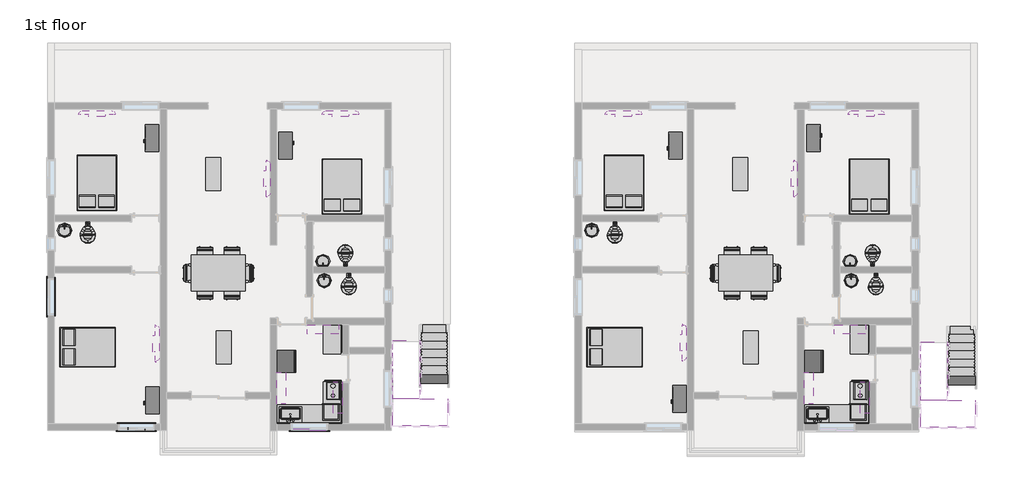
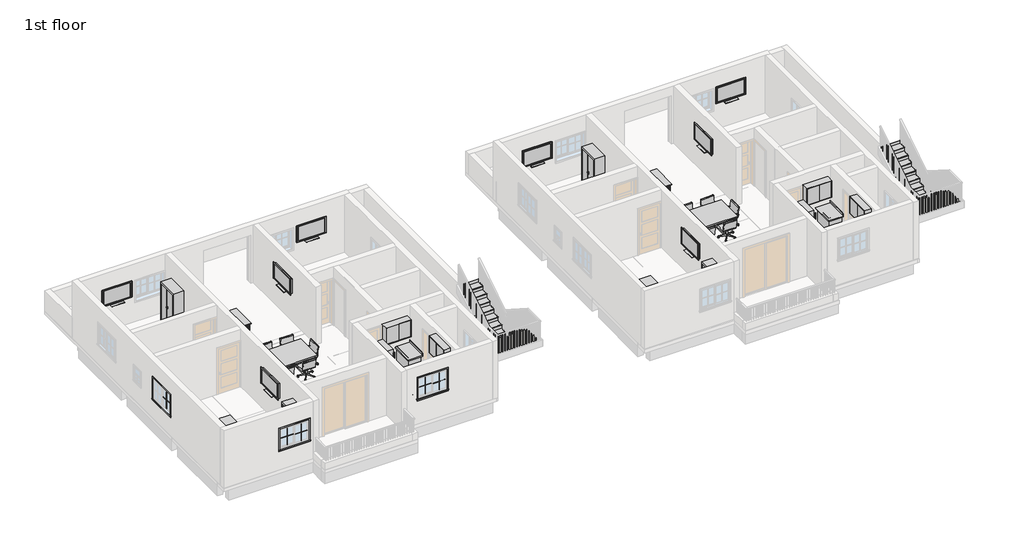
# One storey, part 7 of 8: 56 furniture elements, 24 proxies, 14 flow terminals, 4 stair flights, 2 slabs.
"""IFC4 building model written with IfcOpenShell, lengths in millimetres."""

from ifc_helpers import new_model, si_unit, origin, place, context, project, spatial, transform, mapped, element, save
from components import proxy_3c1fa1d0, proxy_caef4acf, muntin_pattern_2x2_muntin_pattern_2x2_0ac132d2, muntin_pattern_2x2_muntin_pattern_2x2_1fb5fae3, proxy_68898770, proxy_19935bb1, trim_window_exterior_flat_with_sill_c4e67c73, trim_window_exterior_flat_with_sill_729ce974, trim_window_interior_flat_picture_frame_cf1733af, trim_window_interior_flat_picture_frame_5593adf3, flow_terminal_4d548711, flow_terminal_a43f4bde, flow_terminal_3100e559, furniture_6369f5ad, furniture_f415afdb, furniture_97fe820d, furniture_b58f7881, furniture_d3d70ab1, chair_task_chair_task_b7f3823b, chair_task_arms_chair_task_arms_fa5a08ef, furniture_47cc8d9a, furniture_d87d408b, furniture_e7d75d8c, furniture_0b81fedb, furniture_74675f9f, furniture_0bcc43ae, upper_cabinet_sliding_double_door_wall_3e092c2a, non_monolithic_landing_27542c2d, non_monolithic_landing_419a9ad9, stair_flight_dc742093, stair_flight_4d250dde, stair_flight_731070e0, stair_flight_a0137449

model = new_model("IFC4")

# Units and contexts
model_context = context("Model", 3, world=origin())
ifc_project = project(units=[si_unit("LENGTHUNIT", "METRE", prefix="MILLI")], contexts=[model_context])

# Site, building, storey
site = spatial("IfcSite", under=ifc_project)
building = spatial("IfcBuilding", under=site)
storey = spatial("IfcBuildingStorey", under=building, Name="1st floor", Elevation=3810.0)

# Proxies
placement = place(None, origin())
proxy_shape = proxy_3c1fa1d0(model_context)
element("IfcBuildingElementProxy", 1, Name="Cook Top-2 Unit : 12\" x 18\" 2", ObjectType="Cook Top-2 Unit : 12\" x 18\" 2", at=placement, inside=storey, context=model_context, shape_type="MappedRepresentation", body=[
    mapped(proxy_shape, transform((-6699.3993763, -3292.5061971, 3810.0), x_axis=(1.0, 0.0, 0.0), y_axis=(0.0, 1.0, 0.0), z_axis=(0.0, 0.0, 1.0))),
])
element("IfcBuildingElementProxy", 2, Name="Cook Top-2 Unit : 12\" x 18\" 2", ObjectType="Cook Top-2 Unit : 12\" x 18\" 2", at=placement, inside=storey, context=model_context, shape_type="MappedRepresentation", body=[
    mapped(proxy_shape, transform((11175.1761273, -3292.5061971, 3810.0), x_axis=(1.0, 0.0, 0.0), y_axis=(0.0, 1.0, 0.0), z_axis=(0.0, 0.0, 1.0))),
])
proxy_2_shape = proxy_caef4acf(model_context)
element("IfcBuildingElementProxy", 3, Name="Cook Top-2 Unit : 16\" x 22\"", ObjectType="Cook Top-2 Unit : 16\" x 22\"", at=placement, inside=storey, context=model_context, shape_type="MappedRepresentation", body=[
    mapped(proxy_2_shape, transform((-6775.5993763, -4038.6311971, 3810.0), x_axis=(1.0, 0.0, 0.0), y_axis=(0.0, 1.0, 0.0), z_axis=(0.0, 0.0, 1.0))),
])
element("IfcBuildingElementProxy", 4, Name="Cook Top-2 Unit : 16\" x 22\"", ObjectType="Cook Top-2 Unit : 16\" x 22\"", at=placement, inside=storey, context=model_context, shape_type="MappedRepresentation", body=[
    mapped(proxy_2_shape, transform((-6864.4993763, -4089.4311971, 3810.0), x_axis=(1.0, 0.0, 0.0), y_axis=(0.0, 1.0, 0.0), z_axis=(0.0, 0.0, 1.0))),
])
element("IfcBuildingElementProxy", 5, Name="Cook Top-2 Unit : 16\" x 22\"", ObjectType="Cook Top-2 Unit : 16\" x 22\"", at=placement, inside=storey, context=model_context, shape_type="MappedRepresentation", body=[
    mapped(proxy_2_shape, transform((-6699.3993763, -3340.1311971, 3810.0), x_axis=(1.0, 0.0, 0.0), y_axis=(0.0, 1.0, 0.0), z_axis=(0.0, 0.0, 1.0))),
])
element("IfcBuildingElementProxy", 6, Name="Cook Top-2 Unit : 16\" x 22\"", ObjectType="Cook Top-2 Unit : 16\" x 22\"", at=placement, inside=storey, context=model_context, shape_type="MappedRepresentation", body=[
    mapped(proxy_2_shape, transform((-6737.4993763, -3556.0311971, 3810.0), x_axis=(1.0, 0.0, 0.0), y_axis=(0.0, 1.0, 0.0), z_axis=(0.0, 0.0, 1.0))),
])
element("IfcBuildingElementProxy", 7, Name="Cook Top-2 Unit : 16\" x 22\"", ObjectType="Cook Top-2 Unit : 16\" x 22\"", at=placement, inside=storey, context=model_context, shape_type="MappedRepresentation", body=[
    mapped(proxy_2_shape, transform((11098.9761273, -4038.6311971, 3810.0), x_axis=(1.0, 0.0, 0.0), y_axis=(0.0, 1.0, 0.0), z_axis=(0.0, 0.0, 1.0))),
])
element("IfcBuildingElementProxy", 8, Name="Cook Top-2 Unit : 16\" x 22\"", ObjectType="Cook Top-2 Unit : 16\" x 22\"", at=placement, inside=storey, context=model_context, shape_type="MappedRepresentation", body=[
    mapped(proxy_2_shape, transform((11010.0761273, -4089.4311971, 3810.0), x_axis=(1.0, 0.0, 0.0), y_axis=(0.0, 1.0, 0.0), z_axis=(0.0, 0.0, 1.0))),
])
element("IfcBuildingElementProxy", 9, Name="Cook Top-2 Unit : 16\" x 22\"", ObjectType="Cook Top-2 Unit : 16\" x 22\"", at=placement, inside=storey, context=model_context, shape_type="MappedRepresentation", body=[
    mapped(proxy_2_shape, transform((11175.1761273, -3340.1311971, 3810.0), x_axis=(1.0, 0.0, 0.0), y_axis=(0.0, 1.0, 0.0), z_axis=(0.0, 0.0, 1.0))),
])
element("IfcBuildingElementProxy", 10, Name="Cook Top-2 Unit : 16\" x 22\"", ObjectType="Cook Top-2 Unit : 16\" x 22\"", at=placement, inside=storey, context=model_context, shape_type="MappedRepresentation", body=[
    mapped(proxy_2_shape, transform((11137.0761273, -3556.0311971, 3810.0), x_axis=(1.0, 0.0, 0.0), y_axis=(0.0, 1.0, 0.0), z_axis=(0.0, 0.0, 1.0))),
])
muntin_pattern_2x2_muntin_pattern_2x2_shape = muntin_pattern_2x2_muntin_pattern_2x2_0ac132d2(model_context)
element("IfcBuildingElementProxy", 11, Name="Muntin Pattern_2x2 : Muntin Pattern_2x2", ObjectType="Muntin Pattern_2x2 : Muntin Pattern_2x2", at=placement, inside=storey, context=model_context, shape_type="MappedRepresentation", body=[
    mapped(muntin_pattern_2x2_muntin_pattern_2x2_shape, transform((-7707.4618763, -4551.3314015, 5035.55), x_axis=(-1.0, 0.0, 0.0), y_axis=(0.0, -1.0, 0.0), z_axis=(0.0, 0.0, 1.0))),
])
element("IfcBuildingElementProxy", 12, Name="Muntin Pattern_2x2 : Muntin Pattern_2x2", ObjectType="Muntin Pattern_2x2 : Muntin Pattern_2x2", at=placement, inside=storey, context=model_context, shape_type="MappedRepresentation", body=[
    mapped(muntin_pattern_2x2_muntin_pattern_2x2_shape, transform((-7139.1368763, -4595.7814015, 5035.55), x_axis=(-1.0, 0.0, 0.0), y_axis=(0.0, -1.0, 0.0), z_axis=(0.0, 0.0, 1.0))),
])
element("IfcBuildingElementProxy", 13, Name="Muntin Pattern_2x2 : Muntin Pattern_2x2", ObjectType="Muntin Pattern_2x2 : Muntin Pattern_2x2", at=placement, inside=storey, context=model_context, shape_type="MappedRepresentation", body=[
    mapped(muntin_pattern_2x2_muntin_pattern_2x2_shape, transform((-13574.8618763, -4551.3314015, 4806.95), x_axis=(-1.0, 0.0, 0.0), y_axis=(0.0, -1.0, 0.0), z_axis=(0.0, 0.0, 1.0))),
])
element("IfcBuildingElementProxy", 14, Name="Muntin Pattern_2x2 : Muntin Pattern_2x2", ObjectType="Muntin Pattern_2x2 : Muntin Pattern_2x2", at=placement, inside=storey, context=model_context, shape_type="MappedRepresentation", body=[
    mapped(muntin_pattern_2x2_muntin_pattern_2x2_shape, transform((-13006.5368763, -4595.7814015, 4806.95), x_axis=(-1.0, 0.0, 0.0), y_axis=(0.0, -1.0, 0.0), z_axis=(0.0, 0.0, 1.0))),
])
muntin_pattern_2x2_muntin_pattern_2x2_2_shape = muntin_pattern_2x2_muntin_pattern_2x2_1fb5fae3(model_context)
element("IfcBuildingElementProxy", 15, Name="Muntin Pattern_2x2 : Muntin Pattern_2x2", ObjectType="Muntin Pattern_2x2 : Muntin Pattern_2x2", at=placement, inside=storey, context=model_context, shape_type="MappedRepresentation", body=[
    mapped(muntin_pattern_2x2_muntin_pattern_2x2_2_shape, transform((-16246.6243763, -355.5689015, 4806.95), x_axis=(0.0, -1.0, 0.0), y_axis=(1.0, 0.0, 0.0), z_axis=(0.0, 0.0, 1.0))),
])
proxy_3_shape = proxy_68898770(model_context)
element("IfcBuildingElementProxy", 16, Name="Oven Single-Built-in : 21\" x 23 1/2\" x 21\"", ObjectType="Oven Single-Built-in : 21\" x 23 1/2\" x 21\"", at=placement, inside=storey, context=model_context, shape_type="MappedRepresentation", body=[
    mapped(proxy_3_shape, transform((-6728.2243036, -3854.6405426, 4622.8), x_axis=(-1.0, 0.0, 0.0), y_axis=(0.0, -1.0, 0.0), z_axis=(0.0, 0.0, 1.0))),
])
element("IfcBuildingElementProxy", 17, Name="Oven Single-Built-in : 21\" x 23 1/2\" x 21\"", ObjectType="Oven Single-Built-in : 21\" x 23 1/2\" x 21\"", at=placement, inside=storey, context=model_context, shape_type="MappedRepresentation", body=[
    mapped(proxy_3_shape, transform((11146.3512, -3854.6405426, 4622.8), x_axis=(-1.0, 0.0, 0.0), y_axis=(0.0, -1.0, 0.0), z_axis=(0.0, 0.0, 1.0))),
])
proxy_4_shape = proxy_19935bb1(model_context)
element("IfcBuildingElementProxy", 18, Name="Refrigerator-Built-in : 30\" x 24\" LH", ObjectType="Refrigerator-Built-in : 30\" x 24\" LH", at=placement, inside=storey, context=model_context, shape_type="MappedRepresentation", body=[
    mapped(proxy_4_shape, transform((-8238.0754048, -2262.1564015, 3810.0), x_axis=(0.0, 1.0, 0.0), y_axis=(-1.0, 0.0, 0.0), z_axis=(0.0, 0.0, 1.0))),
])
element("IfcBuildingElementProxy", 19, Name="Refrigerator-Built-in : 30\" x 24\" LH", ObjectType="Refrigerator-Built-in : 30\" x 24\" LH", at=placement, inside=storey, context=model_context, shape_type="MappedRepresentation", body=[
    mapped(proxy_4_shape, transform((9636.5000988, -2262.1564015, 3810.0), x_axis=(0.0, 1.0, 0.0), y_axis=(-1.0, 0.0, 0.0), z_axis=(0.0, 0.0, 1.0))),
])
trim_window_exterior_flat_with_sill_shape = trim_window_exterior_flat_with_sill_c4e67c73(model_context)
element("IfcBuildingElementProxy", 20, Name="Trim-Window-Exterior-Flat : with Sill", ObjectType="Trim-Window-Exterior-Flat : with Sill", at=placement, inside=storey, context=model_context, shape_type="MappedRepresentation", body=[
    mapped(trim_window_exterior_flat_with_sill_shape, transform((-7423.2993763, -4605.3064015, 5867.4), x_axis=(1.0, 0.0, 0.0), y_axis=(0.0, 0.0, 1.0), z_axis=(0.0, -1.0, 0.0))),
])
element("IfcBuildingElementProxy", 21, Name="Trim-Window-Exterior-Flat : with Sill", ObjectType="Trim-Window-Exterior-Flat : with Sill", at=placement, inside=storey, context=model_context, shape_type="MappedRepresentation", body=[
    mapped(trim_window_exterior_flat_with_sill_shape, transform((-13290.6993763, -4605.3064015, 5638.8), x_axis=(1.0, 0.0, 0.0), y_axis=(0.0, 0.0, 1.0), z_axis=(0.0, -1.0, 0.0))),
])
trim_window_exterior_flat_with_sill_2_shape = trim_window_exterior_flat_with_sill_729ce974(model_context)
element("IfcBuildingElementProxy", 22, Name="Trim-Window-Exterior-Flat : with Sill", ObjectType="Trim-Window-Exterior-Flat : with Sill", at=placement, inside=storey, context=model_context, shape_type="MappedRepresentation", body=[
    mapped(trim_window_exterior_flat_with_sill_2_shape, transform((-16300.5993763, -71.4064015, 5638.8), x_axis=(0.0, 1.0, 0.0), y_axis=(0.0, 0.0, -1.0), z_axis=(-1.0, 0.0, 0.0))),
])
trim_window_interior_flat_picture_frame_shape = trim_window_interior_flat_picture_frame_cf1733af(model_context)
element("IfcBuildingElementProxy", 23, Name="Trim-Window-Interior-Flat : Picture Frame", ObjectType="Trim-Window-Interior-Flat : Picture Frame", at=placement, inside=storey, context=model_context, shape_type="MappedRepresentation", body=[
    mapped(trim_window_interior_flat_picture_frame_shape, transform((-13290.6993763, -4376.7064015, 5638.8), x_axis=(-1.0, 0.0, 0.0), y_axis=(0.0, 0.0, 1.0), z_axis=(0.0, 1.0, 0.0))),
])
trim_window_interior_flat_picture_frame_2_shape = trim_window_interior_flat_picture_frame_5593adf3(model_context)
element("IfcBuildingElementProxy", 24, Name="Trim-Window-Interior-Flat : Picture Frame", ObjectType="Trim-Window-Interior-Flat : Picture Frame", at=placement, inside=storey, context=model_context, shape_type="MappedRepresentation", body=[
    mapped(trim_window_interior_flat_picture_frame_2_shape, transform((-16071.9993763, -71.4064015, 5638.8), x_axis=(0.0, -1.0, 0.0), y_axis=(0.0, 0.0, -1.0), z_axis=(1.0, 0.0, 0.0))),
])

# Flow terminals
flow_terminal_shape = flow_terminal_4d548711(model_context)
element("IfcFlowTerminal", 25, ObjectType="Sink Kitchen-Single : 30\" x 21\"", at=placement, inside=storey, context=model_context, shape_type="MappedRepresentation", body=[
    mapped(flow_terminal_shape, transform((-8055.3101357, -4069.5610004, 3810.0), x_axis=(-1.0, 0.0, 0.0), y_axis=(0.0, -1.0, 0.0), z_axis=(0.0, 0.0, 1.0))),
])
element("IfcFlowTerminal", 26, ObjectType="Sink Kitchen-Single : 30\" x 21\"", at=placement, inside=storey, context=model_context, shape_type="MappedRepresentation", body=[
    mapped(flow_terminal_shape, transform((9819.2653679, -4069.5610004, 3810.0), x_axis=(-1.0, 0.0, 0.0), y_axis=(0.0, -1.0, 0.0), z_axis=(0.0, 0.0, 1.0))),
])
flow_terminal_2_shape = flow_terminal_a43f4bde(model_context)
element("IfcFlowTerminal", 27, ObjectType="Sink Vanity-Round : 19\" x 19\"", at=placement, inside=storey, context=model_context, shape_type="MappedRepresentation", body=[
    mapped(flow_terminal_2_shape, transform((-15825.7511169, 2099.027665, 3810.0), x_axis=(1.0, 0.0, 0.0), y_axis=(0.0, 1.0, 0.0), z_axis=(0.0, 0.0, 1.0))),
])
element("IfcFlowTerminal", 28, ObjectType="Sink Vanity-Round : 19\" x 19\"", at=placement, inside=storey, context=model_context, shape_type="MappedRepresentation", body=[
    mapped(flow_terminal_2_shape, transform((-6868.8660625, 1205.7175518, 3810.0), x_axis=(-0.999964486635994, 0.008427660815032186, 0.0), y_axis=(-0.008427660815032186, -0.999964486635994, 0.0), z_axis=(0.0, 0.0, 1.0))),
])
element("IfcFlowTerminal", 29, ObjectType="Sink Vanity-Round : 19\" x 19\"", at=placement, inside=storey, context=model_context, shape_type="MappedRepresentation", body=[
    mapped(flow_terminal_2_shape, transform((-7024.6511169, 390.0887767, 3810.0), x_axis=(1.0, 0.0, 0.0), y_axis=(0.0, 1.0, 0.0), z_axis=(0.0, 0.0, 1.0))),
])
element("IfcFlowTerminal", 30, ObjectType="Sink Vanity-Round : 19\" x 19\"", at=placement, inside=storey, context=model_context, shape_type="MappedRepresentation", body=[
    mapped(flow_terminal_2_shape, transform((2048.8243868, 2099.027665, 3810.0), x_axis=(1.0, 0.0, 0.0), y_axis=(0.0, 1.0, 0.0), z_axis=(0.0, 0.0, 1.0))),
])
element("IfcFlowTerminal", 31, ObjectType="Sink Vanity-Round : 19\" x 19\"", at=placement, inside=storey, context=model_context, shape_type="MappedRepresentation", body=[
    mapped(flow_terminal_2_shape, transform((11005.7094411, 1205.7175518, 3810.0), x_axis=(-0.999964486635994, 0.008427660815032186, 0.0), y_axis=(-0.008427660815032186, -0.999964486635994, 0.0), z_axis=(0.0, 0.0, 1.0))),
])
element("IfcFlowTerminal", 32, ObjectType="Sink Vanity-Round : 19\" x 19\"", at=placement, inside=storey, context=model_context, shape_type="MappedRepresentation", body=[
    mapped(flow_terminal_2_shape, transform((10849.9243868, 390.0887767, 3810.0), x_axis=(1.0, 0.0, 0.0), y_axis=(0.0, 1.0, 0.0), z_axis=(0.0, 0.0, 1.0))),
])
flow_terminal_3_shape = flow_terminal_3100e559(model_context)
element("IfcFlowTerminal", 33, ObjectType="Toilet-Commercial-Wall-3D : 15\" Seat Height", at=placement, inside=storey, context=model_context, shape_type="MappedRepresentation", body=[
    mapped(flow_terminal_3_shape, transform((-5684.8962225, 842.9935985, 3810.0), x_axis=(-1.0, 0.0, 0.0), y_axis=(0.0, -1.0, 0.0), z_axis=(0.0, 0.0, 1.0))),
])
element("IfcFlowTerminal", 34, ObjectType="Toilet-Commercial-Wall-3D : 15\" Seat Height", at=placement, inside=storey, context=model_context, shape_type="MappedRepresentation", body=[
    mapped(flow_terminal_3_shape, transform((-6609.0025301, 842.9935985, 3810.0), x_axis=(1.0, 0.0, 0.0), y_axis=(0.0, 1.0, 0.0), z_axis=(0.0, 0.0, 1.0))),
])
element("IfcFlowTerminal", 35, ObjectType="Toilet-Commercial-Wall-3D : 15\" Seat Height", at=placement, inside=storey, context=model_context, shape_type="MappedRepresentation", body=[
    mapped(flow_terminal_3_shape, transform((-14536.7962225, 2595.5935985, 3810.0), x_axis=(-1.0, 0.0, 0.0), y_axis=(0.0, -1.0, 0.0), z_axis=(0.0, 0.0, 1.0))),
])
element("IfcFlowTerminal", 36, ObjectType="Toilet-Commercial-Wall-3D : 15\" Seat Height", at=placement, inside=storey, context=model_context, shape_type="MappedRepresentation", body=[
    mapped(flow_terminal_3_shape, transform((12189.6792812, 842.9935985, 3810.0), x_axis=(-1.0, 0.0, 0.0), y_axis=(0.0, -1.0, 0.0), z_axis=(0.0, 0.0, 1.0))),
])
element("IfcFlowTerminal", 37, ObjectType="Toilet-Commercial-Wall-3D : 15\" Seat Height", at=placement, inside=storey, context=model_context, shape_type="MappedRepresentation", body=[
    mapped(flow_terminal_3_shape, transform((11265.5729735, 842.9935985, 3810.0), x_axis=(1.0, 0.0, 0.0), y_axis=(0.0, 1.0, 0.0), z_axis=(0.0, 0.0, 1.0))),
])
element("IfcFlowTerminal", 38, ObjectType="Toilet-Commercial-Wall-3D : 15\" Seat Height", at=placement, inside=storey, context=model_context, shape_type="MappedRepresentation", body=[
    mapped(flow_terminal_3_shape, transform((3337.7792812, 2595.5935985, 3810.0), x_axis=(-1.0, 0.0, 0.0), y_axis=(0.0, -1.0, 0.0), z_axis=(0.0, 0.0, 1.0))),
])

# Furniture
furniture_shape = furniture_6369f5ad(model_context)
element("IfcFurniture", 39, ObjectType="Base Cabinet-Acid Storage Unit : 30\" 2", at=placement, inside=storey, context=model_context, shape_type="MappedRepresentation", body=[
    mapped(furniture_shape, transform((-6343.7993763, -3202.2686966, 3810.0), x_axis=(0.0, -1.0, 0.0), y_axis=(1.0, 0.0, 0.0), z_axis=(0.0, 0.0, 1.0))),
])
element("IfcFurniture", 40, ObjectType="Base Cabinet-Acid Storage Unit : 30\" 2", at=placement, inside=storey, context=model_context, shape_type="MappedRepresentation", body=[
    mapped(furniture_shape, transform((11530.7761273, -3202.2686966, 3810.0), x_axis=(0.0, -1.0, 0.0), y_axis=(1.0, 0.0, 0.0), z_axis=(0.0, 0.0, 1.0))),
])
furniture_2_shape = furniture_f415afdb(model_context)
element("IfcFurniture", 41, ObjectType="Base Cabinet-Combo01 : 30\" 2", at=placement, inside=storey, context=model_context, shape_type="MappedRepresentation", body=[
    mapped(furniture_2_shape, transform((-6318.3993763, -1386.1686966, 3810.0), x_axis=(0.0, -1.0, 0.0), y_axis=(1.0, 0.0, 0.0), z_axis=(0.0, 0.0, 1.0))),
])
element("IfcFurniture", 42, ObjectType="Base Cabinet-Combo01 : 30\" 2", at=placement, inside=storey, context=model_context, shape_type="MappedRepresentation", body=[
    mapped(furniture_2_shape, transform((11556.1761273, -1386.1686966, 3810.0), x_axis=(0.0, -1.0, 0.0), y_axis=(1.0, 0.0, 0.0), z_axis=(0.0, 0.0, 1.0))),
])
furniture_3_shape = furniture_97fe820d(model_context)
element("IfcFurniture", 43, ObjectType="Base Cabinet-Corner Unit-Square : 36\"", at=placement, inside=storey, context=model_context, shape_type="MappedRepresentation", body=[
    mapped(furniture_3_shape, transform((-6318.3993763, -3849.9686966, 3810.0), x_axis=(0.0, -1.0, 0.0), y_axis=(1.0, 0.0, 0.0), z_axis=(0.0, 0.0, 1.0))),
])
element("IfcFurniture", 44, ObjectType="Base Cabinet-Corner Unit-Square : 36\"", at=placement, inside=storey, context=model_context, shape_type="MappedRepresentation", body=[
    mapped(furniture_3_shape, transform((11556.1761273, -3849.9686966, 3810.0), x_axis=(0.0, -1.0, 0.0), y_axis=(1.0, 0.0, 0.0), z_axis=(0.0, 0.0, 1.0))),
])
furniture_4_shape = furniture_b58f7881(model_context)
element("IfcFurniture", 45, ObjectType="Bed-Box : Double 53\" x 74\"", at=placement, inside=storey, context=model_context, shape_type="MappedRepresentation", body=[
    mapped(furniture_4_shape, transform((-14292.2379089, 3557.6185064, 3810.0), x_axis=(-1.0, 0.0, 0.0), y_axis=(0.0, -1.0, 0.0), z_axis=(0.0, 0.0, 1.0))),
])
element("IfcFurniture", 46, ObjectType="Bed-Box : Double 53\" x 74\"", at=placement, inside=storey, context=model_context, shape_type="MappedRepresentation", body=[
    mapped(furniture_4_shape, transform((-15182.9191795, -2125.0588605, 3810.0), x_axis=(0.0, 1.0, 0.0), y_axis=(-1.0, 0.0, 0.0), z_axis=(0.0, 0.0, 1.0))),
])
element("IfcFurniture", 47, ObjectType="Bed-Box : Double 53\" x 74\"", at=placement, inside=storey, context=model_context, shape_type="MappedRepresentation", body=[
    mapped(furniture_4_shape, transform((-5979.2469173, 3433.3274594, 3810.0), x_axis=(-1.0, 0.0, 0.0), y_axis=(0.0, -1.0, 0.0), z_axis=(0.0, 0.0, 1.0))),
])
element("IfcFurniture", 48, ObjectType="Bed-Box : Double 53\" x 74\"", at=placement, inside=storey, context=model_context, shape_type="MappedRepresentation", body=[
    mapped(furniture_4_shape, transform((3582.3375948, 3557.6185064, 3810.0), x_axis=(-1.0, 0.0, 0.0), y_axis=(0.0, -1.0, 0.0), z_axis=(0.0, 0.0, 1.0))),
])
element("IfcFurniture", 49, ObjectType="Bed-Box : Double 53\" x 74\"", at=placement, inside=storey, context=model_context, shape_type="MappedRepresentation", body=[
    mapped(furniture_4_shape, transform((2691.6563242, -2125.0588605, 3810.0), x_axis=(0.0, 1.0, 0.0), y_axis=(-1.0, 0.0, 0.0), z_axis=(0.0, 0.0, 1.0))),
])
element("IfcFurniture", 50, ObjectType="Bed-Box : Double 53\" x 74\"", at=placement, inside=storey, context=model_context, shape_type="MappedRepresentation", body=[
    mapped(furniture_4_shape, transform((11895.3285864, 3433.3274594, 3810.0), x_axis=(-1.0, 0.0, 0.0), y_axis=(0.0, -1.0, 0.0), z_axis=(0.0, 0.0, 1.0))),
])
furniture_5_shape = furniture_d3d70ab1(model_context)
element("IfcFurniture", 51, ObjectType="Cabinet-Storage : 36\" x 18\" x 72\"", at=placement, inside=storey, context=model_context, shape_type="MappedRepresentation", body=[
    mapped(furniture_5_shape, transform((-12757.2993763, 5305.7833167, 3810.0), x_axis=(0.0, -1.0, 0.0), y_axis=(1.0, 0.0, 0.0), z_axis=(0.0, 0.0, 1.0))),
])
element("IfcFurniture", 52, ObjectType="Cabinet-Storage : 36\" x 18\" x 72\"", at=placement, inside=storey, context=model_context, shape_type="MappedRepresentation", body=[
    mapped(furniture_5_shape, transform((-8236.2515468, 5059.3935985, 3810.0), x_axis=(0.0, 1.0, 0.0), y_axis=(-1.0, 0.0, 0.0), z_axis=(0.0, 0.0, 1.0))),
])
element("IfcFurniture", 53, ObjectType="Cabinet-Storage : 36\" x 18\" x 72\"", at=placement, inside=storey, context=model_context, shape_type="MappedRepresentation", body=[
    mapped(furniture_5_shape, transform((-12748.5420807, -3590.3671413, 3810.0), x_axis=(0.0, -1.0, 0.0), y_axis=(1.0, 0.0, 0.0), z_axis=(0.0, 0.0, 1.0))),
])
element("IfcFurniture", 54, ObjectType="Cabinet-Storage : 36\" x 18\" x 72\"", at=placement, inside=storey, context=model_context, shape_type="MappedRepresentation", body=[
    mapped(furniture_5_shape, transform((4992.1783017, 5059.3935985, 3810.0), x_axis=(0.0, -1.0, 0.0), y_axis=(1.0, 0.0, 0.0), z_axis=(0.0, 0.0, 1.0))),
])
element("IfcFurniture", 55, ObjectType="Cabinet-Storage : 36\" x 18\" x 72\"", at=placement, inside=storey, context=model_context, shape_type="MappedRepresentation", body=[
    mapped(furniture_5_shape, transform((5126.8930163, -3538.5064015, 3810.0), x_axis=(0.0, -1.0, 0.0), y_axis=(1.0, 0.0, 0.0), z_axis=(0.0, 0.0, 1.0))),
])
element("IfcFurniture", 56, ObjectType="Cabinet-Storage : 36\" x 18\" x 72\"", at=placement, inside=storey, context=model_context, shape_type="MappedRepresentation", body=[
    mapped(furniture_5_shape, transform((9660.8090799, 5305.7833167, 3810.0), x_axis=(0.0, 1.0, 0.0), y_axis=(-1.0, 0.0, 0.0), z_axis=(0.0, 0.0, 1.0))),
])
chair_task_chair_task_shape = chair_task_chair_task_b7f3823b(model_context)
element("IfcFurniture", 57, ObjectType="Chair-Task : Chair-Task", at=placement, inside=storey, context=model_context, shape_type="MappedRepresentation", body=[
    mapped(chair_task_chair_task_shape, transform((-9911.2085566, 1357.2395001, 3810.0), x_axis=(-1.0, 0.0, 0.0), y_axis=(0.0, -1.0, 0.0), z_axis=(0.0, 0.0, 1.0))),
])
element("IfcFurniture", 58, ObjectType="Chair-Task : Chair-Task", at=placement, inside=storey, context=model_context, shape_type="MappedRepresentation", body=[
    mapped(chair_task_chair_task_shape, transform((-10193.190196, 100.1476968, 3810.0), x_axis=(1.0, 0.0, 0.0), y_axis=(0.0, 1.0, 0.0), z_axis=(0.0, 0.0, 1.0))),
])
element("IfcFurniture", 59, ObjectType="Chair-Task : Chair-Task", at=placement, inside=storey, context=model_context, shape_type="MappedRepresentation", body=[
    mapped(chair_task_chair_task_shape, transform((-10825.6085566, 1357.2395001, 3810.0), x_axis=(-1.0, 0.0, 0.0), y_axis=(0.0, -1.0, 0.0), z_axis=(0.0, 0.0, 1.0))),
])
element("IfcFurniture", 60, ObjectType="Chair-Task : Chair-Task", at=placement, inside=storey, context=model_context, shape_type="MappedRepresentation", body=[
    mapped(chair_task_chair_task_shape, transform((-11107.590196, 100.1476968, 3810.0), x_axis=(1.0, 0.0, 0.0), y_axis=(0.0, 1.0, 0.0), z_axis=(0.0, 0.0, 1.0))),
])
element("IfcFurniture", 61, ObjectType="Chair-Task : Chair-Task", at=placement, inside=storey, context=model_context, shape_type="MappedRepresentation", body=[
    mapped(chair_task_chair_task_shape, transform((7963.366947, 1357.2395001, 3810.0), x_axis=(-1.0, 0.0, 0.0), y_axis=(0.0, -1.0, 0.0), z_axis=(0.0, 0.0, 1.0))),
])
element("IfcFurniture", 62, ObjectType="Chair-Task : Chair-Task", at=placement, inside=storey, context=model_context, shape_type="MappedRepresentation", body=[
    mapped(chair_task_chair_task_shape, transform((7681.3853077, 100.1476968, 3810.0), x_axis=(1.0, 0.0, 0.0), y_axis=(0.0, 1.0, 0.0), z_axis=(0.0, 0.0, 1.0))),
])
element("IfcFurniture", 63, ObjectType="Chair-Task : Chair-Task", at=placement, inside=storey, context=model_context, shape_type="MappedRepresentation", body=[
    mapped(chair_task_chair_task_shape, transform((7048.966947, 1357.2395001, 3810.0), x_axis=(-1.0, 0.0, 0.0), y_axis=(0.0, -1.0, 0.0), z_axis=(0.0, 0.0, 1.0))),
])
element("IfcFurniture", 64, ObjectType="Chair-Task : Chair-Task", at=placement, inside=storey, context=model_context, shape_type="MappedRepresentation", body=[
    mapped(chair_task_chair_task_shape, transform((6766.9853077, 100.1476968, 3810.0), x_axis=(1.0, 0.0, 0.0), y_axis=(0.0, 1.0, 0.0), z_axis=(0.0, 0.0, 1.0))),
])
chair_task_arms_chair_task_arms_shape = chair_task_arms_chair_task_arms_fa5a08ef(model_context)
element("IfcFurniture", 65, ObjectType="Chair-Task Arms : Chair-Task Arms", at=placement, inside=storey, context=model_context, shape_type="MappedRepresentation", body=[
    mapped(chair_task_arms_chair_task_arms_shape, transform((-11442.7452779, 869.6844182, 3810.0), x_axis=(0.0, -1.0, 0.0), y_axis=(1.0, 0.0, 0.0), z_axis=(0.0, 0.0, 1.0))),
])
element("IfcFurniture", 66, ObjectType="Chair-Task Arms : Chair-Task Arms", at=placement, inside=storey, context=model_context, shape_type="MappedRepresentation", body=[
    mapped(chair_task_arms_chair_task_arms_shape, transform((-9576.0534746, 587.7027788, 3810.0), x_axis=(0.0, 1.0, 0.0), y_axis=(-1.0, 0.0, 0.0), z_axis=(0.0, 0.0, 1.0))),
])
element("IfcFurniture", 67, ObjectType="Chair-Task Arms : Chair-Task Arms", at=placement, inside=storey, context=model_context, shape_type="MappedRepresentation", body=[
    mapped(chair_task_arms_chair_task_arms_shape, transform((6431.8302257, 869.6844182, 3810.0), x_axis=(0.0, -1.0, 0.0), y_axis=(1.0, 0.0, 0.0), z_axis=(0.0, 0.0, 1.0))),
])
element("IfcFurniture", 68, ObjectType="Chair-Task Arms : Chair-Task Arms", at=placement, inside=storey, context=model_context, shape_type="MappedRepresentation", body=[
    mapped(chair_task_arms_chair_task_arms_shape, transform((8298.522029, 587.7027788, 3810.0), x_axis=(0.0, 1.0, 0.0), y_axis=(-1.0, 0.0, 0.0), z_axis=(0.0, 0.0, 1.0))),
])
furniture_6_shape = furniture_47cc8d9a(model_context)
element("IfcFurniture", 69, ObjectType="Counter Top : 24\" Depth", at=placement, inside=storey, context=model_context, shape_type="MappedRepresentation", body=[
    mapped(furniture_6_shape, transform((-6318.3993763, -2224.3686966, 3810.0), x_axis=(0.0, -1.0, 0.0), y_axis=(1.0, 0.0, 0.0), z_axis=(0.0, 0.0, 1.0))),
])
element("IfcFurniture", 70, ObjectType="Counter Top : 24\" Depth", at=placement, inside=storey, context=model_context, shape_type="MappedRepresentation", body=[
    mapped(furniture_6_shape, transform((11556.1761273, -2224.3686966, 3810.0), x_axis=(0.0, -1.0, 0.0), y_axis=(1.0, 0.0, 0.0), z_axis=(0.0, 0.0, 1.0))),
])
furniture_7_shape = furniture_d87d408b(model_context)
element("IfcFurniture", 71, ObjectType="Counter Top : 24\" Depth", at=placement, inside=storey, context=model_context, shape_type="MappedRepresentation", body=[
    mapped(furniture_7_shape, transform((-6318.3993763, -4167.4686966, 3810.0), x_axis=(0.0, -1.0, 0.0), y_axis=(1.0, 0.0, 0.0), z_axis=(0.0, 0.0, 1.0))),
])
element("IfcFurniture", 72, ObjectType="Counter Top : 24\" Depth", at=placement, inside=storey, context=model_context, shape_type="MappedRepresentation", body=[
    mapped(furniture_7_shape, transform((11556.1761273, -4167.4686966, 3810.0), x_axis=(0.0, -1.0, 0.0), y_axis=(1.0, 0.0, 0.0), z_axis=(0.0, 0.0, 1.0))),
])
furniture_8_shape = furniture_e7d75d8c(model_context)
element("IfcFurniture", 73, ObjectType="Counter Top w Sink Hole : 24\" Depth", at=placement, inside=storey, context=model_context, shape_type="MappedRepresentation", body=[
    mapped(furniture_8_shape, transform((-7518.8616714, -4376.7064015, 3810.0), x_axis=(-1.0, 0.0, 0.0), y_axis=(0.0, -1.0, 0.0), z_axis=(0.0, 0.0, 1.0))),
])
element("IfcFurniture", 74, ObjectType="Counter Top w Sink Hole : 24\" Depth", at=placement, inside=storey, context=model_context, shape_type="MappedRepresentation", body=[
    mapped(furniture_8_shape, transform((10355.7138323, -4376.7064015, 3810.0), x_axis=(-1.0, 0.0, 0.0), y_axis=(0.0, -1.0, 0.0), z_axis=(0.0, 0.0, 1.0))),
])
furniture_9_shape = furniture_0b81fedb(model_context)
element("IfcFurniture", 75, ObjectType="TV - Flat Screen : 50\"", at=placement, inside=storey, context=model_context, shape_type="MappedRepresentation", body=[
    mapped(furniture_9_shape, transform((-8815.3379999, 3937.8490843, 5029.2), x_axis=(0.0, -1.0, 0.0), y_axis=(1.0, 0.0, 0.0), z_axis=(0.0, 0.0, 1.0))),
])
element("IfcFurniture", 76, ObjectType="TV - Flat Screen : 50\"", at=placement, inside=storey, context=model_context, shape_type="MappedRepresentation", body=[
    mapped(furniture_9_shape, transform((-14627.4458537, 6186.2439145, 5029.2), x_axis=(1.0, 0.0, 0.0), y_axis=(0.0, 1.0, 0.0), z_axis=(0.0, 0.0, 1.0))),
])
element("IfcFurniture", 77, ObjectType="TV - Flat Screen : 50\"", at=placement, inside=storey, context=model_context, shape_type="MappedRepresentation", body=[
    mapped(furniture_9_shape, transform((-12581.2234035, -1662.8509157, 5029.2), x_axis=(0.0, -1.0, 0.0), y_axis=(1.0, 0.0, 0.0), z_axis=(0.0, 0.0, 1.0))),
])
element("IfcFurniture", 78, ObjectType="TV - Flat Screen : 50\"", at=placement, inside=storey, context=model_context, shape_type="MappedRepresentation", body=[
    mapped(furniture_9_shape, transform((-6365.2548621, 6186.2439145, 5029.2), x_axis=(1.0, 0.0, 0.0), y_axis=(0.0, 1.0, 0.0), z_axis=(0.0, 0.0, 1.0))),
])
element("IfcFurniture", 79, ObjectType="TV - Flat Screen : 50\"", at=placement, inside=storey, context=model_context, shape_type="MappedRepresentation", body=[
    mapped(furniture_9_shape, transform((9059.2375037, 3937.8490843, 5029.2), x_axis=(0.0, -1.0, 0.0), y_axis=(1.0, 0.0, 0.0), z_axis=(0.0, 0.0, 1.0))),
])
element("IfcFurniture", 80, ObjectType="TV - Flat Screen : 50\"", at=placement, inside=storey, context=model_context, shape_type="MappedRepresentation", body=[
    mapped(furniture_9_shape, transform((3226.0357212, 6186.2439145, 5029.2), x_axis=(1.0, 0.0, 0.0), y_axis=(0.0, 1.0, 0.0), z_axis=(0.0, 0.0, 1.0))),
])
element("IfcFurniture", 81, ObjectType="TV - Flat Screen : 50\"", at=placement, inside=storey, context=model_context, shape_type="MappedRepresentation", body=[
    mapped(furniture_9_shape, transform((11458.5206415, 6186.2439145, 5029.2), x_axis=(1.0, 0.0, 0.0), y_axis=(0.0, 1.0, 0.0), z_axis=(0.0, 0.0, 1.0))),
])
element("IfcFurniture", 82, ObjectType="TV - Flat Screen : 50\"", at=placement, inside=storey, context=model_context, shape_type="MappedRepresentation", body=[
    mapped(furniture_9_shape, transform((5293.3521002, -1637.4509157, 5029.2), x_axis=(0.0, -1.0, 0.0), y_axis=(1.0, 0.0, 0.0), z_axis=(0.0, 0.0, 1.0))),
])
furniture_10_shape = furniture_74675f9f(model_context)
element("IfcFurniture", 83, ObjectType="Table-Coffee Mission : 44\" x 20\"", at=placement, inside=storey, context=model_context, shape_type="MappedRepresentation", body=[
    mapped(furniture_10_shape, transform((-10683.4908966, 4085.6049296, 3810.0), x_axis=(0.0, 1.0, 0.0), y_axis=(-1.0, 0.0, 0.0), z_axis=(0.0, 0.0, 1.0))),
])
element("IfcFurniture", 84, ObjectType="Table-Coffee Mission : 44\" x 20\"", at=placement, inside=storey, context=model_context, shape_type="MappedRepresentation", body=[
    mapped(furniture_10_shape, transform((-10337.6073421, -1785.9064015, 3810.0), x_axis=(0.0, 1.0, 0.0), y_axis=(-1.0, 0.0, 0.0), z_axis=(0.0, 0.0, 1.0))),
])
element("IfcFurniture", 85, ObjectType="Table-Coffee Mission : 44\" x 20\"", at=placement, inside=storey, context=model_context, shape_type="MappedRepresentation", body=[
    mapped(furniture_10_shape, transform((7191.084607, 4085.6049296, 3810.0), x_axis=(0.0, 1.0, 0.0), y_axis=(-1.0, 0.0, 0.0), z_axis=(0.0, 0.0, 1.0))),
])
element("IfcFurniture", 86, ObjectType="Table-Coffee Mission : 44\" x 20\"", at=placement, inside=storey, context=model_context, shape_type="MappedRepresentation", body=[
    mapped(furniture_10_shape, transform((7536.9681616, -1785.9064015, 3810.0), x_axis=(0.0, 1.0, 0.0), y_axis=(-1.0, 0.0, 0.0), z_axis=(0.0, 0.0, 1.0))),
])
furniture_11_shape = furniture_0bcc43ae(model_context)
element("IfcFurniture", 87, ObjectType="Table-Conference2 w Chairs : 48\" x 144\"", at=placement, inside=storey, context=model_context, shape_type="MappedRepresentation", body=[
    mapped(furniture_11_shape, transform((-10509.3993763, 728.6935985, 3810.0), x_axis=(1.0, 0.0, 0.0), y_axis=(0.0, 1.0, 0.0), z_axis=(0.0, 0.0, 1.0))),
])
element("IfcFurniture", 88, ObjectType="Table-Conference2 w Chairs : 48\" x 144\"", at=placement, inside=storey, context=model_context, shape_type="MappedRepresentation", body=[
    mapped(furniture_11_shape, transform((7365.1761273, 728.6935985, 3810.0), x_axis=(1.0, 0.0, 0.0), y_axis=(0.0, 1.0, 0.0), z_axis=(0.0, 0.0, 1.0))),
])
upper_cabinet_sliding_double_door_wall_shape = upper_cabinet_sliding_double_door_wall_3e092c2a(model_context)
element("IfcFurniture", 89, ObjectType="Upper Cabinet-Sliding Double Door-Wall", at=placement, inside=storey, context=model_context, shape_type="MappedRepresentation", body=[
    mapped(upper_cabinet_sliding_double_door_wall_shape, transform((-6204.0993763, -3530.1775643, 4152.9), x_axis=(0.0, 1.0, 0.0), y_axis=(-1.0, 0.0, 0.0), z_axis=(0.0, 0.0, 1.0))),
])
element("IfcFurniture", 90, ObjectType="Upper Cabinet-Sliding Double Door-Wall", at=placement, inside=storey, context=model_context, shape_type="MappedRepresentation", body=[
    mapped(upper_cabinet_sliding_double_door_wall_shape, transform((-6936.3282135, -909.6064015, 3810.0), x_axis=(-1.0, 0.0, 0.0), y_axis=(0.0, -1.0, 0.0), z_axis=(0.0, 0.0, 1.0))),
])
element("IfcFurniture", 91, ObjectType="Upper Cabinet-Sliding Double Door-Wall", at=placement, inside=storey, context=model_context, shape_type="MappedRepresentation", body=[
    mapped(upper_cabinet_sliding_double_door_wall_shape, transform((-8642.4993763, -3140.4352387, 3810.0), x_axis=(0.0, -1.0, 0.0), y_axis=(1.0, 0.0, 0.0), z_axis=(0.0, 0.0, 1.0))),
])
element("IfcFurniture", 92, ObjectType="Upper Cabinet-Sliding Double Door-Wall", at=placement, inside=storey, context=model_context, shape_type="MappedRepresentation", body=[
    mapped(upper_cabinet_sliding_double_door_wall_shape, transform((11670.4761273, -3530.1775643, 4152.9), x_axis=(0.0, 1.0, 0.0), y_axis=(-1.0, 0.0, 0.0), z_axis=(0.0, 0.0, 1.0))),
])
element("IfcFurniture", 93, ObjectType="Upper Cabinet-Sliding Double Door-Wall", at=placement, inside=storey, context=model_context, shape_type="MappedRepresentation", body=[
    mapped(upper_cabinet_sliding_double_door_wall_shape, transform((10938.2472901, -909.6064015, 3810.0), x_axis=(-1.0, 0.0, 0.0), y_axis=(0.0, -1.0, 0.0), z_axis=(0.0, 0.0, 1.0))),
])
element("IfcFurniture", 94, ObjectType="Upper Cabinet-Sliding Double Door-Wall", at=placement, inside=storey, context=model_context, shape_type="MappedRepresentation", body=[
    mapped(upper_cabinet_sliding_double_door_wall_shape, transform((9232.0761273, -3140.4352387, 3810.0), x_axis=(0.0, -1.0, 0.0), y_axis=(1.0, 0.0, 0.0), z_axis=(0.0, 0.0, 1.0))),
])

# Slabs
non_monolithic_landing_shape = non_monolithic_landing_27542c2d(model_context)
element("IfcSlab", 95, ObjectType="Non-Monolithic Landing", at=placement, inside=storey, context=model_context, shape_type="MappedRepresentation", body=[
    mapped(non_monolithic_landing_shape, transform((0.0, 0.0, 0.0), x_axis=(1.0, 0.0, 0.0), y_axis=(0.0, 1.0, 0.0), z_axis=(0.0, 0.0, 1.0))),
])
non_monolithic_landing_2_shape = non_monolithic_landing_419a9ad9(model_context)
element("IfcSlab", 96, ObjectType="Non-Monolithic Landing", at=placement, inside=storey, context=model_context, shape_type="MappedRepresentation", body=[
    mapped(non_monolithic_landing_2_shape, transform((0.0, 0.0, 0.0), x_axis=(1.0, 0.0, 0.0), y_axis=(0.0, 1.0, 0.0), z_axis=(0.0, 0.0, 1.0))),
])

# Stair flights
stair_flight_shape = stair_flight_dc742093(model_context)
element("IfcStairFlight", 97, ObjectType="2\" Tread 1\" Nosing 1/4\" Riser", at=placement, inside=storey, context=model_context, shape_type="MappedRepresentation", body=[
    mapped(stair_flight_shape, transform((0.0, 0.0, 0.0), x_axis=(1.0, 0.0, 0.0), y_axis=(0.0, 1.0, 0.0), z_axis=(0.0, 0.0, 1.0))),
])
stair_flight_2_shape = stair_flight_4d250dde(model_context)
element("IfcStairFlight", 98, ObjectType="2\" Tread 1\" Nosing 1/4\" Riser", at=placement, inside=storey, context=model_context, shape_type="MappedRepresentation", body=[
    mapped(stair_flight_2_shape, transform((0.0, 0.0, 0.0), x_axis=(1.0, 0.0, 0.0), y_axis=(0.0, 1.0, 0.0), z_axis=(0.0, 0.0, 1.0))),
])
stair_flight_3_shape = stair_flight_731070e0(model_context)
element("IfcStairFlight", 99, ObjectType="2\" Tread 1\" Nosing 1/4\" Riser", at=placement, inside=storey, context=model_context, shape_type="MappedRepresentation", body=[
    mapped(stair_flight_3_shape, transform((0.0, 0.0, 0.0), x_axis=(1.0, 0.0, 0.0), y_axis=(0.0, 1.0, 0.0), z_axis=(0.0, 0.0, 1.0))),
])
stair_flight_4_shape = stair_flight_a0137449(model_context)
element("IfcStairFlight", 100, ObjectType="2\" Tread 1\" Nosing 1/4\" Riser", at=placement, inside=storey, context=model_context, shape_type="MappedRepresentation", body=[
    mapped(stair_flight_4_shape, transform((0.0, 0.0, 0.0), x_axis=(1.0, 0.0, 0.0), y_axis=(0.0, 1.0, 0.0), z_axis=(0.0, 0.0, 1.0))),
])

save(model, "model.ifc")

# Revit data of these elements
# Type "Cook Top-2 Unit : 12\" x 18\" 2"
#   Assembly Code = "E1090400"
#   Counter Height = 3' - 0"
#   Depth = 2' - 0"
#   Width = 1' - 6"
#   Burner Material = Metal - Chrome
#   Cooktop Material = Metal - Steel, Polished
#   Default Elevation = 0
# Type "Cook Top-2 Unit : 16\" x 22\""
#   Assembly Code = "E1090400"
#   Counter Height = 2' - 7"
#   Depth = 1' - 10"
#   Width = 1' - 4"
#   Burner Material = Metal - Chrome
#   Cooktop Material = Metal - Steel, Polished
#   Default Elevation = 0
# Type "Muntin Pattern_2x2 : Muntin Pattern_2x2"
#   Width [instance default] = 4' - 0"
#   Thickness = 0' - 0 1/2"
#   Height [instance default] = 4' - 0"
#   Distance = 0' - 0 3/4"
#   Interior Material [instance default] = none
#   Exterior Material [instance default] = none
#   Default Elevation = 0
# Type "Oven Single-Built-in : 21\" x 23 1/2\" x 21\""
#   Label = "OVEN"
#   Assembly Code = "E1090400"
#   Depth = 1' - 9"
#   Height = 1' - 11 1/2"
#   Install Height = 0' - 9 1/2"
#   Width = 1' - 9 1/2"
#   Oven Material = Metal - Stainless Steel, Polished
#   Default Elevation = 0
# Type "Refrigerator-Built-in : 30\" x 24\" LH"
#   Assembly Code = "E1090400"
#   Depth = 2' - 0"
#   Handle = 0' - 0 1/4"
#   Height = 7' - 0"
#   Top Door Height = 5' - 0"
#   Width = 2' - 5 1/2"
#   Material = Metal - Paint Finish - Ivory,Glossy
#   Default Elevation = 0
# Type "Trim-Window-Exterior-Flat : with Sill"
#   Trim Width = 0' - 2 1/4"
#   Trim Thickness_Picture Frame = 0' - 1 1/4"
#   Trim Thickness_with Sill = 0' - 0 3/4"
#   Sill Thickness = 0' - 1 1/4"
#   Opening Width [instance default] = 2' - 0"
#   Opening Height [instance default] = 3' - 0"
#   Default Elevation = 4' - 0"
#   Sill = yes
#   Picture Frame = no
#   Trim Material [instance default] = none
# Type "Trim-Window-Interior-Flat : Picture Frame"
#   Trim Thickness_Picture Frame = 0' - 1 1/4"
#   Trim Width = 0' - 2 1/4"
#   Trim Thickness_with Sill = 0' - 0 3/4"
#   Sill Thickness = 0' - 1 1/4"
#   Opening Width [instance default] = 2' - 0"
#   Opening Height [instance default] = 3' - 0"
#   Default Elevation = 4' - 0"
#   Sill = no
#   Picture Frame = yes
#   Trim Material [instance default] = none
# Type "Sink Kitchen-Single : 30\" x 21\""
#   Assembly Code = "D2010410"
#   Counter Height = 3' - 0"
#   Depth = 1' - 9"
#   Width = 2' - 6"
#   Faucet Material = Steel, Polished
#   Sink Material = Steel, Polished
#   Default Elevation = 0
# Type "Sink Vanity-Round : 19\" x 19\""
#   Assembly Code = "D2010400"
#   Top Of Counter = 2' - 7"
#   Basin Material = Porcelain, Linen
#   Faucet Material = Steel, Polished
#   Default Elevation = 0
# Type "Toilet-Commercial-Wall-3D : 15\" Seat Height"
#   Assembly Code = "D2010110"
#   Mounting Height = 1' - 3"
#   Piping Material = Steel, Polished
#   Toilet - Bowl Material = Porcelain, Ivory
#   Toilet - Seat Material = Laminate, Ivory, Matte
#   Default Elevation = 0
# Type "Base Cabinet-Acid Storage Unit : 30\" 2"
#   Depth = 1' - 10"
#   Height = 2' - 11 3/4"
#   Toe Depth = 0' - 3"
#   Toe Height = 0' - 3 1/2"
#   Width = 2' - 0"
#   Default Elevation = 0
# Type "Base Cabinet-Combo01 : 30\" 2"
#   Depth = 1' - 10"
#   Height = 2' - 11 3/4"
#   Toe Depth = 0' - 3"
#   Toe Height = 0' - 3 1/2"
#   Width = 3' - 0"
#   Default Elevation = 0
# Type "Base Cabinet-Corner Unit-Square : 36\""
#   Assembly Code = "C1030410"
#   Depth = 2' - 0"
#   Height = 2' - 10 1/2"
#   Toe Depth = 0' - 3"
#   Toe Height = 0' - 3 1/2"
#   Width = 3' - 0"
#   Cabinet Material = Cabinets
#   Door/Drawer Material = Cabinets
#   Handle Material = Cabinets - Handles
#   Default Elevation = 0
# Type "Bed-Box : Double 53\" x 74\""
#   Assembly Code = "E2020200"
#   Length = 6' - 2"
#   Width = 4' - 5"
#   Frame Material = Birch
#   Mattress Material = Linen, White
#   Default Elevation = 0
# Type "Cabinet-Storage : 36\" x 18\" x 72\""
#   Assembly Code = "E2020200"
#   Depth = 1' - 6"
#   Height = 6' - 0"
#   Width = 3' - 0"
#   Material = Metal - Steel
#   Default Elevation = 0
# Type "Chair-Task : Chair-Task"
#   Assembly Code = "E2020200"
#   Base Material = Plastic - Black
#   Caster Material = Plastic - Black
#   Seat/Back Material = Textile - Slate Blue
#   Default Elevation = 0
# Type "Chair-Task Arms : Chair-Task Arms"
#   Assembly Code = "E2020200"
#   Base Material = Plastic - Black
#   Caster Material = Plastic - Black
#   Seat/Back Material = Textile - Slate Blue
#   Default Elevation = 0
# Type "Counter Top : 24\" Depth"
#   Assembly Code = "C1030400"
#   Counter Thickness = 0' - 1 1/2"
#   Depth = 2' - 1"
#   Height = 3' - 0"
#   Length [instance default] = 8' - 0"
#   Counter Top Material = none
#   Default Elevation = 0
# Type "Counter Top w Sink Hole : 24\" Depth"
#   Assembly Code = "C1030400"
#   Counter Thickness = 0' - 1 1/2"
#   Depth = 2' - 1"
#   Height = 3' - 0"
#   Length [instance default] = 8' - 0"
#   Sink Location [instance default] = 2' - 0"
#   Sink Location To Wall [instance default] = 0' - 6"
#   Sink Opening Depth [instance default] = 1' - 3"
#   Sink Opening Width [instance default] = 2' - 3"
#   Counter Top Material = none
#   Default Elevation = 0
# Type "TV - Flat Screen : 50\""
#   SinAng = 0' - 0.0193"
#   L = 3' - 7.57782"
#   H = 2' - 0.51477"
#   Thickness = 0' - 4.33071"
#   Diagonal = 4' - 2"
#   CosAng = 0' - 0.03431"
#   Stand [instance default] = yes
#   Default Elevation = 0
# Type "Table-Coffee Mission : 44\" x 20\""
#   Assembly Code = "E2020200"
#   Height = 1' - 5"
#   Length = 3' - 8"
#   Width = 1' - 8"
#   Material = Wood - Mahogany
#   Default Elevation = 0
# Type "Table-Conference2 w Chairs : 48\" x 144\""
#   Assembly Code = "E2020200"
#   Description = "Seating 12-14"
#   Height = 2' - 6"
#   Length = 6' - 0"
#   Width = 4' - 0"
#   Number Of Chairs One Side = 2
#   Number Of Chairs = 6
#   Material = Wood - Cherry
#   Default Elevation = 0
# Type "Upper Cabinet-Sliding Double Door-Wall"
#   Depth = 1' - 0"
#   Height = 2' - 6"
#   Top Of Cabinet = 7' - 0"
#   Width = 3' - 6"
#   Default Elevation = 0
# Elements 1, 2 (IfcBuildingElementProxy, "Cook Top-2 Unit : 12\" x 18\" 2")
#   Phase Created = New Construction
#   Materials on its faces: "Metal - Steel, Polished", "Metal - Chrome"
# Elements 3, 4, 5, 6, 7, 8, 9, 10 (IfcBuildingElementProxy, "Cook Top-2 Unit : 16\" x 22\"")
#   Phase Created = New Construction
#   Materials on its faces: "Metal - Steel, Polished", "Metal - Chrome"
# Elements 11, 12, 13, 14, 15 (IfcBuildingElementProxy, "Muntin Pattern_2x2 : Muntin Pattern_2x2")
#   Width = 1' - 8 5/8"
#   Height = 2' - 6 1/4"
#   Interior Material = Wood - Stained
#   Exterior Material = Clad - White
#   Phase Created = New Construction
#   Materials on its faces: "Clad - White", "Wood - Stained"
# Elements 16, 17 (IfcBuildingElementProxy, "Oven Single-Built-in : 21\" x 23 1/2\" x 21\"")
#   Phase Created = New Construction
#   Materials on its faces: "Metal - Steel", "Metal - Stainless Steel, Polished", "Glass"
# Elements 18, 19 (IfcBuildingElementProxy, "Refrigerator-Built-in : 30\" x 24\" LH")
#   Phase Created = New Construction
#   Materials on its faces: "Metal - Paint Finish - Ivory,Glossy", "Metal - Chrome"
# Elements 20, 21, 22 (IfcBuildingElementProxy, "Trim-Window-Exterior-Flat : with Sill")
#   Opening Width = 4' - 0"
#   Opening Height = 3' - 0"
#   Trim Material = Clad - White
#   Phase Created = New Construction
#   Materials on its faces: "Clad - White"
# Elements 23, 24 (IfcBuildingElementProxy, "Trim-Window-Interior-Flat : Picture Frame")
#   Opening Width = 4' - 0"
#   Opening Height = 3' - 0"
#   Trim Material = Wood - Stained
#   Phase Created = New Construction
#   Materials on its faces: "Wood - Stained"
# Element 25 (IfcFlowTerminal, "Sink Kitchen-Single : 30\" x 21\"")
#   Mark = "23"
#   Phase Created = New Construction
#   Materials on its faces: "Steel, Polished"
# Element 26 (IfcFlowTerminal, "Sink Kitchen-Single : 30\" x 21\"")
#   Mark = "31"
#   Phase Created = New Construction
#   Materials on its faces: "Steel, Polished"
# Element 27 (IfcFlowTerminal, "Sink Vanity-Round : 19\" x 19\"")
#   Mark = "24"
#   Phase Created = New Construction
#   Materials on its faces: "Porcelain, Linen", "Steel, Polished"
# Element 28 (IfcFlowTerminal, "Sink Vanity-Round : 19\" x 19\"")
#   Mark = "25"
#   Phase Created = New Construction
#   Materials on its faces: "Porcelain, Linen", "Steel, Polished"
# Element 29 (IfcFlowTerminal, "Sink Vanity-Round : 19\" x 19\"")
#   Mark = "26"
#   Phase Created = New Construction
#   Materials on its faces: "Porcelain, Linen", "Steel, Polished"
# Element 30 (IfcFlowTerminal, "Sink Vanity-Round : 19\" x 19\"")
#   Mark = "32"
#   Phase Created = New Construction
#   Materials on its faces: "Porcelain, Linen", "Steel, Polished"
# Element 31 (IfcFlowTerminal, "Sink Vanity-Round : 19\" x 19\"")
#   Mark = "33"
#   Phase Created = New Construction
#   Materials on its faces: "Porcelain, Linen", "Steel, Polished"
# Element 32 (IfcFlowTerminal, "Sink Vanity-Round : 19\" x 19\"")
#   Mark = "34"
#   Phase Created = New Construction
#   Materials on its faces: "Porcelain, Linen", "Steel, Polished"
# Element 33 (IfcFlowTerminal, "Toilet-Commercial-Wall-3D : 15\" Seat Height")
#   Mark = "27"
#   Phase Created = New Construction
#   Materials on its faces: "Laminate, Ivory, Matte", "Porcelain, Ivory", "Steel, Polished"
# Element 34 (IfcFlowTerminal, "Toilet-Commercial-Wall-3D : 15\" Seat Height")
#   Mark = "28"
#   Phase Created = New Construction
#   Materials on its faces: "Laminate, Ivory, Matte", "Porcelain, Ivory", "Steel, Polished"
# Element 35 (IfcFlowTerminal, "Toilet-Commercial-Wall-3D : 15\" Seat Height")
#   Mark = "29"
#   Phase Created = New Construction
#   Materials on its faces: "Laminate, Ivory, Matte", "Porcelain, Ivory", "Steel, Polished"
# Element 36 (IfcFlowTerminal, "Toilet-Commercial-Wall-3D : 15\" Seat Height")
#   Mark = "35"
#   Phase Created = New Construction
#   Materials on its faces: "Laminate, Ivory, Matte", "Porcelain, Ivory", "Steel, Polished"
# Element 37 (IfcFlowTerminal, "Toilet-Commercial-Wall-3D : 15\" Seat Height")
#   Mark = "36"
#   Phase Created = New Construction
#   Materials on its faces: "Laminate, Ivory, Matte", "Porcelain, Ivory", "Steel, Polished"
# Element 38 (IfcFlowTerminal, "Toilet-Commercial-Wall-3D : 15\" Seat Height")
#   Mark = "37"
#   Phase Created = New Construction
#   Materials on its faces: "Laminate, Ivory, Matte", "Porcelain, Ivory", "Steel, Polished"
# Elements 39, 40 (IfcFurniture, "Base Cabinet-Acid Storage Unit : 30\" 2")
#   Phase Created = New Construction
#   Materials on its faces: "Cabinet"
# Elements 41, 42 (IfcFurniture, "Base Cabinet-Combo01 : 30\" 2")
#   Phase Created = New Construction
#   Materials on its faces: "Cabinet"
# Elements 43, 44 (IfcFurniture, "Base Cabinet-Corner Unit-Square : 36\"")
#   Phase Created = New Construction
#   Materials on its faces: "Cabinets", "Cabinets - Handles"
# Elements 45, 46, 47, 48, 49, 50 (IfcFurniture, "Bed-Box : Double 53\" x 74\"")
#   Phase Created = New Construction
#   Materials on its faces: "Birch", "Linen, White"
# Elements 51, 52, 53, 54, 55, 56 (IfcFurniture, "Cabinet-Storage : 36\" x 18\" x 72\"")
#   Phase Created = New Construction
#   Materials on its faces: "Metal - Steel", "Metal - Chrome"
# Elements 57, 58, 59, 60, 61, 62, 63, 64 (IfcFurniture, "Chair-Task : Chair-Task")
#   Phase Created = New Construction
#   Materials on its faces: "Plastic - Black", "Textile - Slate Blue"
# Elements 65, 66, 67, 68 (IfcFurniture, "Chair-Task Arms : Chair-Task Arms")
#   Phase Created = New Construction
#   Materials on its faces: "Plastic - Black", "Textile - Slate Blue"
# Elements 69, 70 (IfcFurniture, "Counter Top : 24\" Depth")
#   Length = 3' - 3"
#   Phase Created = New Construction
#   Materials on its faces: "Counter Top"
# Elements 71, 72 (IfcFurniture, "Counter Top : 24\" Depth")
#   Length = 4' - 7 1/2"
#   Phase Created = New Construction
#   Materials on its faces: "Counter Top"
# Elements 73, 74 (IfcFurniture, "Counter Top w Sink Hole : 24\" Depth")
#   Sink Opening Width = 2' - 3"
#   Sink Opening Depth = 1' - 3"
#   Sink Location To Wall = 0' - 6"
#   Sink Location = 5' - 9"
#   Length = 7' - 3"
#   Phase Created = New Construction
#   Materials on its faces: "Counter Top"
# Elements 75, 76, 77, 78, 79, 80, 81, 82 (IfcFurniture, "TV - Flat Screen : 50\"")
#   Stand = yes
#   Phase Created = New Construction
#   Materials on its faces: "TV - Black", "TV - Glass", "TV - Screen"
# Elements 83, 84, 85, 86 (IfcFurniture, "Table-Coffee Mission : 44\" x 20\"")
#   Phase Created = New Construction
#   Materials on its faces: "Wood - Mahogany"
# Elements 87, 88 (IfcFurniture, "Table-Conference2 w Chairs : 48\" x 144\"")
#   Phase Created = New Construction
#   Materials on its faces: "Wood - Cherry"
# Elements 89, 90, 91, 92, 93, 94 (IfcFurniture, "Upper Cabinet-Sliding Double Door-Wall")
#   Phase Created = New Construction
#   Materials on its faces: "Cabinet", "Glass"
# Elements 95, 96 (IfcSlab, "Non-Monolithic Landing")
#   Phase Created = New Construction
# Elements 97, 98, 99, 100 (IfcStairFlight, "2\" Tread 1\" Nosing 1/4\" Riser")
#   Phase Created = New Construction
# Materials
#   "Metal - Chrome": colour RGB 17 17 17, transparency 0
#   "Metal - Steel, Polished": colour RGB 127 127 127, transparency 0
#   "Metal - Stainless Steel, Polished": colour RGB 215 215 215, transparency 0
#   "Metal - Paint Finish - Ivory,Glossy": colour RGB 247 247 239, transparency 0
#   "Steel, Polished": class "Metal", colour RGB 57 57 57, transparency 0, Description = "Polished steel", Cost = 0
#   "Porcelain, Linen": class "Ceramic", colour RGB 249 239 230, transparency 0, Description = "Porcelain, linen", Cost = 0
#   "Porcelain, Ivory": class "Ceramic", colour RGB 247 247 239, transparency 0, Description = "Porcelain, ivory", Cost = 0
#   "Laminate, Ivory, Matte": class "Plastic", colour RGB 247 247 239, transparency 0, Description = "Plastic Laminate - Ivory, Matte", Cost = 0
#   "Cabinets": colour RGB 249 249 249, transparency 0
#   "Cabinets - Handles": colour RGB 57 57 57, transparency 0
#   "Birch": class "Wood", colour RGB 224 178 126, transparency 0, Description = "Betula Alleghaniensis", Cost = 0
#   "Linen, White": class "Textile", colour RGB 247 247 239, transparency 0, Description = "Linen, white", Cost = 0
#   "Metal - Steel": colour RGB 247 247 247, transparency 0
#   "Plastic - Black": colour RGB 0 0 0, transparency 0.7
#   "Textile - Slate Blue": colour RGB 98 102 118, transparency 0
#   "Wood - Mahogany": colour RGB 138 86 45, transparency 0
#   "Wood - Cherry": colour RGB 151 75 0, transparency 0
#   "Clad - White": class "Wood", colour RGB 242 242 238, transparency 0, Cost = 0
#   "Wood - Stained": class "Wood", colour RGB 224 178 126, transparency 0, Cost = 0
#   "Glass": class "Glass", colour RGB 0 128 192, transparency 0.75, Description = "Soda Lime Glass", Cost = 0
#   "Cabinet": colour RGB 204 122 2, transparency 0
#   "Counter Top": class "Wood", colour RGB 226 177 128, transparency 0
#   "TV - Black": colour RGB 49 49 49, transparency 0
#   "TV - Glass": colour RGB 157 157 157, transparency 0.9
#   "TV - Screen": colour RGB 0 0 0, transparency 0
